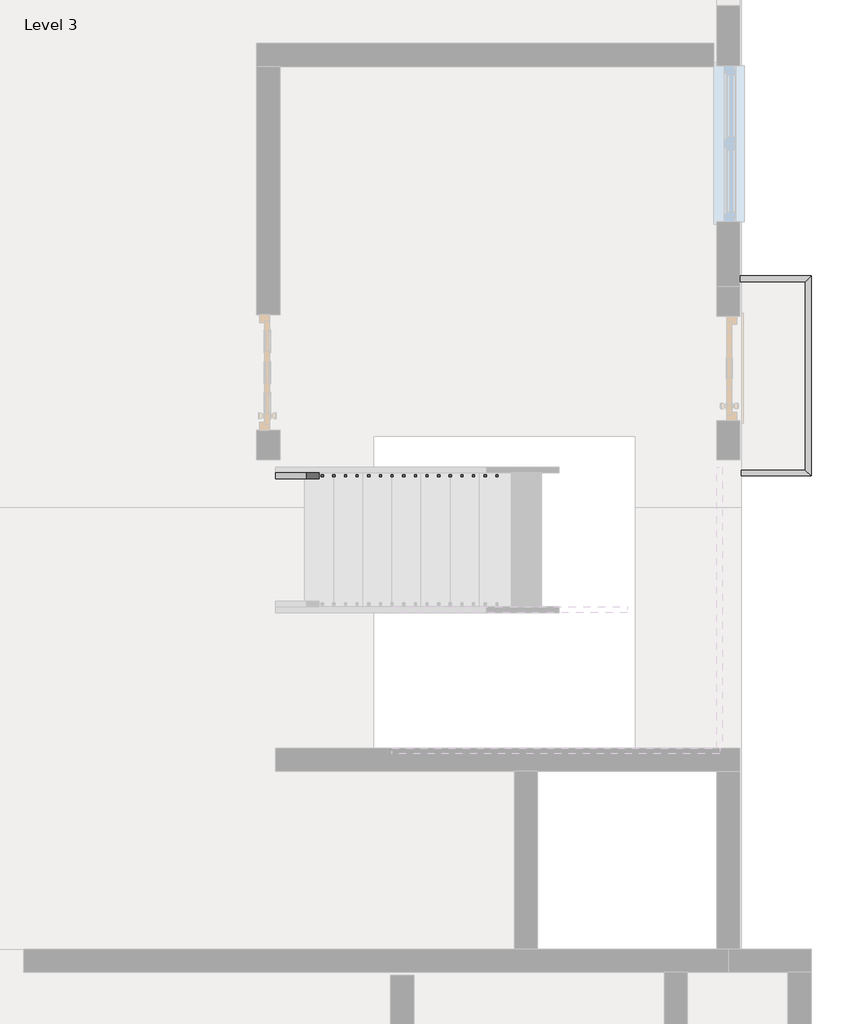
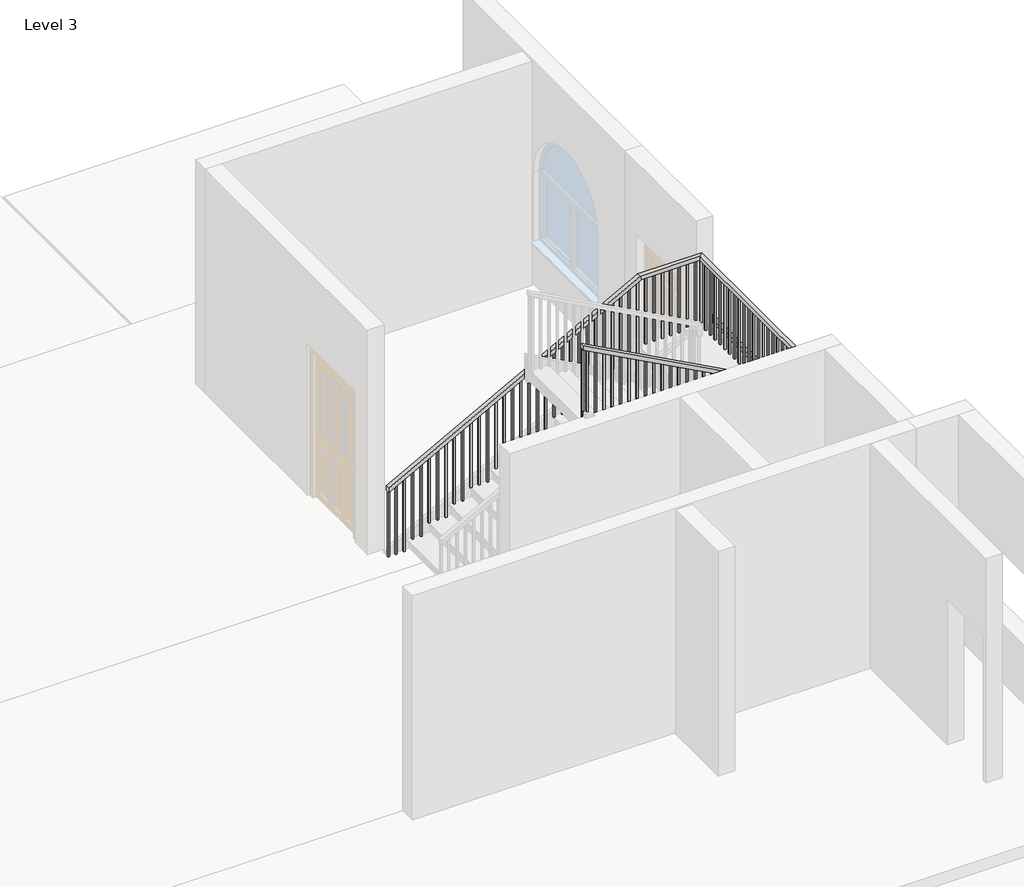
# One storey, part 6 of 7: 2 railings.
"""IFC4 building model written with IfcOpenShell, lengths in millimetres."""

from ifc_helpers import new_model, si_unit, frame, origin, place, context, project, spatial, polyline, outline, extrude, faceted_brep, element, save

model = new_model("IFC4")

# Units and contexts
model_context = context("Model", 3, world=origin())
ifc_project = project(units=[si_unit("LENGTHUNIT", "METRE", prefix="MILLI")], contexts=[model_context])

# Site, building, storey
site = spatial("IfcSite", under=ifc_project)
building = spatial("IfcBuilding", under=site)
storey = spatial("IfcBuildingStorey", under=building, Name="Level 3", Elevation=6096.0)

# Railings
placement = place(None, origin())
element("IfcRailing", 1, ObjectType="Handrail - Rectangular", at=placement, inside=storey, context=model_context, shape_type="SolidModel", body=[
    faceted_brep([(5863.1890963, 3183.81308, 7010.4), (5863.1890963, 3183.81308, 6959.6), (5863.1890963, 3133.01308, 6959.6), (5863.1890963, 3133.01308, 7010.4), (6485.4890963, 3183.81308, 7010.4), (6485.4890963, 3183.81308, 6959.6), (6434.6890963, 3133.01308, 6959.6), (6434.6890963, 3133.01308, 7010.4), (6485.4890963, 1439.3962251, 7010.4), (6485.4890963, 1439.3962251, 6959.6), (6434.6890963, 1490.1962251, 6959.6), (6434.6890963, 1490.1962251, 7010.4), (5875.8890963, 1439.3962251, 7010.4), (5875.8890963, 1490.1962251, 7010.4), (5875.8890963, 1490.1962251, 6959.6), (5875.8890963, 1439.3962251, 6959.6)], [[[0, 1, 2, 3]], [[1, 0, 4, 5]], [[2, 1, 5, 6]], [[3, 2, 6, 7]], [[0, 3, 7, 4]], [[5, 4, 8, 9]], [[6, 5, 9, 10]], [[7, 6, 10, 11]], [[4, 7, 11, 8]], [[12, 13, 14, 15]], [[9, 8, 12, 15]], [[10, 9, 15, 14]], [[11, 10, 14, 13]], [[8, 11, 13, 12]]]),
    extrude(outline(polyline([(5961.6140963, 1474.3212251), (5961.6140963, 1455.2712251), (5942.5640963, 1455.2712251), (5942.5640963, 1474.3212251), (5961.6140963, 1474.3212251)])), frame((0.0, 0.0, 6096.0), z_axis=(0.0, 0.0, 1.0), x_axis=(1.0, 0.0, 0.0)), (0.0, 0.0, 1.0), 863.6),
    extrude(outline(polyline([(6063.2140963, 1474.3212251), (6063.2140963, 1455.2712251), (6044.1640963, 1455.2712251), (6044.1640963, 1474.3212251), (6063.2140963, 1474.3212251)])), frame((0.0, 0.0, 6096.0), z_axis=(0.0, 0.0, 1.0), x_axis=(1.0, 0.0, 0.0)), (0.0, 0.0, 1.0), 863.6),
    extrude(outline(polyline([(6164.8140963, 1474.3212251), (6164.8140963, 1455.2712251), (6145.7640963, 1455.2712251), (6145.7640963, 1474.3212251), (6164.8140963, 1474.3212251)])), frame((0.0, 0.0, 6096.0), z_axis=(0.0, 0.0, 1.0), x_axis=(1.0, 0.0, 0.0)), (0.0, 0.0, 1.0), 863.6),
    extrude(outline(polyline([(6266.4140963, 1474.3212251), (6266.4140963, 1455.2712251), (6247.3640963, 1455.2712251), (6247.3640963, 1474.3212251), (6266.4140963, 1474.3212251)])), frame((0.0, 0.0, 6096.0), z_axis=(0.0, 0.0, 1.0), x_axis=(1.0, 0.0, 0.0)), (0.0, 0.0, 1.0), 863.6),
    extrude(outline(polyline([(6368.0140963, 1474.3212251), (6368.0140963, 1455.2712251), (6348.9640963, 1455.2712251), (6348.9640963, 1474.3212251), (6368.0140963, 1474.3212251)])), frame((0.0, 0.0, 6096.0), z_axis=(0.0, 0.0, 1.0), x_axis=(1.0, 0.0, 0.0)), (0.0, 0.0, 1.0), 863.6),
    extrude(outline(polyline([(6450.5640963, 1542.33808), (6469.6140963, 1542.33808), (6469.6140963, 1523.28808), (6450.5640963, 1523.28808), (6450.5640963, 1542.33808)])), frame((0.0, 0.0, 6096.0), z_axis=(0.0, 0.0, 1.0), x_axis=(1.0, 0.0, 0.0)), (0.0, 0.0, 1.0), 863.6),
    extrude(outline(polyline([(6450.5640963, 1643.93808), (6469.6140963, 1643.93808), (6469.6140963, 1624.88808), (6450.5640963, 1624.88808), (6450.5640963, 1643.93808)])), frame((0.0, 0.0, 6096.0), z_axis=(0.0, 0.0, 1.0), x_axis=(1.0, 0.0, 0.0)), (0.0, 0.0, 1.0), 863.6),
    extrude(outline(polyline([(6450.5640963, 1745.53808), (6469.6140963, 1745.53808), (6469.6140963, 1726.48808), (6450.5640963, 1726.48808), (6450.5640963, 1745.53808)])), frame((0.0, 0.0, 6096.0), z_axis=(0.0, 0.0, 1.0), x_axis=(1.0, 0.0, 0.0)), (0.0, 0.0, 1.0), 863.6),
    extrude(outline(polyline([(6450.5640963, 1847.13808), (6469.6140963, 1847.13808), (6469.6140963, 1828.08808), (6450.5640963, 1828.08808), (6450.5640963, 1847.13808)])), frame((0.0, 0.0, 6096.0), z_axis=(0.0, 0.0, 1.0), x_axis=(1.0, 0.0, 0.0)), (0.0, 0.0, 1.0), 863.6),
    extrude(outline(polyline([(6450.5640963, 1948.73808), (6469.6140963, 1948.73808), (6469.6140963, 1929.68808), (6450.5640963, 1929.68808), (6450.5640963, 1948.73808)])), frame((0.0, 0.0, 6096.0), z_axis=(0.0, 0.0, 1.0), x_axis=(1.0, 0.0, 0.0)), (0.0, 0.0, 1.0), 863.6),
    extrude(outline(polyline([(6450.5640963, 2050.33808), (6469.6140963, 2050.33808), (6469.6140963, 2031.28808), (6450.5640963, 2031.28808), (6450.5640963, 2050.33808)])), frame((0.0, 0.0, 6096.0), z_axis=(0.0, 0.0, 1.0), x_axis=(1.0, 0.0, 0.0)), (0.0, 0.0, 1.0), 863.6),
    extrude(outline(polyline([(6450.5640963, 2151.93808), (6469.6140963, 2151.93808), (6469.6140963, 2132.88808), (6450.5640963, 2132.88808), (6450.5640963, 2151.93808)])), frame((0.0, 0.0, 6096.0), z_axis=(0.0, 0.0, 1.0), x_axis=(1.0, 0.0, 0.0)), (0.0, 0.0, 1.0), 863.6),
    extrude(outline(polyline([(6450.5640963, 2253.53808), (6469.6140963, 2253.53808), (6469.6140963, 2234.48808), (6450.5640963, 2234.48808), (6450.5640963, 2253.53808)])), frame((0.0, 0.0, 6096.0), z_axis=(0.0, 0.0, 1.0), x_axis=(1.0, 0.0, 0.0)), (0.0, 0.0, 1.0), 863.6),
    extrude(outline(polyline([(6450.5640963, 2355.13808), (6469.6140963, 2355.13808), (6469.6140963, 2336.08808), (6450.5640963, 2336.08808), (6450.5640963, 2355.13808)])), frame((0.0, 0.0, 6096.0), z_axis=(0.0, 0.0, 1.0), x_axis=(1.0, 0.0, 0.0)), (0.0, 0.0, 1.0), 863.6),
    extrude(outline(polyline([(6450.5640963, 2456.73808), (6469.6140963, 2456.73808), (6469.6140963, 2437.68808), (6450.5640963, 2437.68808), (6450.5640963, 2456.73808)])), frame((0.0, 0.0, 6096.0), z_axis=(0.0, 0.0, 1.0), x_axis=(1.0, 0.0, 0.0)), (0.0, 0.0, 1.0), 863.6),
    extrude(outline(polyline([(6450.5640963, 2558.33808), (6469.6140963, 2558.33808), (6469.6140963, 2539.28808), (6450.5640963, 2539.28808), (6450.5640963, 2558.33808)])), frame((0.0, 0.0, 6096.0), z_axis=(0.0, 0.0, 1.0), x_axis=(1.0, 0.0, 0.0)), (0.0, 0.0, 1.0), 863.6),
    extrude(outline(polyline([(6450.5640963, 2659.93808), (6469.6140963, 2659.93808), (6469.6140963, 2640.88808), (6450.5640963, 2640.88808), (6450.5640963, 2659.93808)])), frame((0.0, 0.0, 6096.0), z_axis=(0.0, 0.0, 1.0), x_axis=(1.0, 0.0, 0.0)), (0.0, 0.0, 1.0), 863.6),
    extrude(outline(polyline([(6450.5640963, 2761.53808), (6469.6140963, 2761.53808), (6469.6140963, 2742.48808), (6450.5640963, 2742.48808), (6450.5640963, 2761.53808)])), frame((0.0, 0.0, 6096.0), z_axis=(0.0, 0.0, 1.0), x_axis=(1.0, 0.0, 0.0)), (0.0, 0.0, 1.0), 863.6),
    extrude(outline(polyline([(6450.5640963, 2863.13808), (6469.6140963, 2863.13808), (6469.6140963, 2844.08808), (6450.5640963, 2844.08808), (6450.5640963, 2863.13808)])), frame((0.0, 0.0, 6096.0), z_axis=(0.0, 0.0, 1.0), x_axis=(1.0, 0.0, 0.0)), (0.0, 0.0, 1.0), 863.6),
    extrude(outline(polyline([(6450.5640963, 2964.73808), (6469.6140963, 2964.73808), (6469.6140963, 2945.68808), (6450.5640963, 2945.68808), (6450.5640963, 2964.73808)])), frame((0.0, 0.0, 6096.0), z_axis=(0.0, 0.0, 1.0), x_axis=(1.0, 0.0, 0.0)), (0.0, 0.0, 1.0), 863.6),
    extrude(outline(polyline([(6450.5640963, 3066.33808), (6469.6140963, 3066.33808), (6469.6140963, 3047.28808), (6450.5640963, 3047.28808), (6450.5640963, 3066.33808)])), frame((0.0, 0.0, 6096.0), z_axis=(0.0, 0.0, 1.0), x_axis=(1.0, 0.0, 0.0)), (0.0, 0.0, 1.0), 863.6),
    extrude(outline(polyline([(6361.6640963, 3148.88808), (6361.6640963, 3167.93808), (6380.7140963, 3167.93808), (6380.7140963, 3148.88808), (6361.6640963, 3148.88808)])), frame((0.0, 0.0, 6096.0), z_axis=(0.0, 0.0, 1.0), x_axis=(1.0, 0.0, 0.0)), (0.0, 0.0, 1.0), 863.6),
    extrude(outline(polyline([(6260.0640963, 3148.88808), (6260.0640963, 3167.93808), (6279.1140963, 3167.93808), (6279.1140963, 3148.88808), (6260.0640963, 3148.88808)])), frame((0.0, 0.0, 6096.0), z_axis=(0.0, 0.0, 1.0), x_axis=(1.0, 0.0, 0.0)), (0.0, 0.0, 1.0), 863.6),
    extrude(outline(polyline([(6158.4640963, 3148.88808), (6158.4640963, 3167.93808), (6177.5140963, 3167.93808), (6177.5140963, 3148.88808), (6158.4640963, 3148.88808)])), frame((0.0, 0.0, 6096.0), z_axis=(0.0, 0.0, 1.0), x_axis=(1.0, 0.0, 0.0)), (0.0, 0.0, 1.0), 863.6),
    extrude(outline(polyline([(6056.8640963, 3148.88808), (6056.8640963, 3167.93808), (6075.9140963, 3167.93808), (6075.9140963, 3148.88808), (6056.8640963, 3148.88808)])), frame((0.0, 0.0, 6096.0), z_axis=(0.0, 0.0, 1.0), x_axis=(1.0, 0.0, 0.0)), (0.0, 0.0, 1.0), 863.6),
    extrude(outline(polyline([(5955.2640963, 3148.88808), (5955.2640963, 3167.93808), (5974.3140963, 3167.93808), (5974.3140963, 3148.88808), (5955.2640963, 3148.88808)])), frame((0.0, 0.0, 6096.0), z_axis=(0.0, 0.0, 1.0), x_axis=(1.0, 0.0, 0.0)), (0.0, 0.0, 1.0), 863.6),
    extrude(outline(polyline([(6450.5640963, 1474.3212251), (6469.6140963, 1474.3212251), (6469.6140963, 1455.2712251), (6450.5640963, 1455.2712251), (6450.5640963, 1474.3212251)])), frame((0.0, 0.0, 6096.0), z_axis=(0.0, 0.0, 1.0), x_axis=(1.0, 0.0, 0.0)), (0.0, 0.0, 1.0), 863.6),
    extrude(outline(polyline([(6450.5640963, 3148.88808), (6450.5640963, 3167.93808), (6469.6140963, 3167.93808), (6469.6140963, 3148.88808), (6450.5640963, 3148.88808)])), frame((0.0, 0.0, 6096.0), z_axis=(0.0, 0.0, 1.0), x_axis=(1.0, 0.0, 0.0)), (0.0, 0.0, 1.0), 863.6),
    extrude(outline(polyline([(5894.9390963, 1474.3212251), (5894.9390963, 1455.2712251), (5875.8890963, 1455.2712251), (5875.8890963, 1474.3212251), (5894.9390963, 1474.3212251)])), frame((0.0, 0.0, 6096.0), z_axis=(0.0, 0.0, 1.0), x_axis=(1.0, 0.0, 0.0)), (0.0, 0.0, 1.0), 863.6),
    extrude(outline(polyline([(5863.1890963, 3148.88808), (5863.1890963, 3167.93808), (5882.2390963, 3167.93808), (5882.2390963, 3148.88808), (5863.1890963, 3148.88808)])), frame((0.0, 0.0, 6096.0), z_axis=(0.0, 0.0, 1.0), x_axis=(1.0, 0.0, 0.0)), (0.0, 0.0, 1.0), 863.6),
])
element("IfcRailing", 2, ObjectType="Handrail - Rectangular", at=placement, inside=storey, context=model_context, shape_type="SolidModel", body=[
    faceted_brep([(1811.8890963, 1464.7962251, 7148.9454545), (1811.8890963, 1464.7962251, 7091.1709673), (1811.8890963, 1413.9962251, 7091.1709673), (1811.8890963, 1413.9962251, 7148.9454545), (4881.0326586, 1464.7962251, 8811.4909091), (4893.9079172, 1464.7962251, 8760.6909091), (4893.9079172, 1413.9962251, 8760.6909091), (4881.0326586, 1413.9962251, 8811.4909091), (5659.9890963, 1464.7962251, 8811.4909091), (5659.9890963, 1464.7962251, 8760.6909091), (5609.1890963, 1413.9962251, 8760.6909091), (5609.1890963, 1413.9962251, 8811.4909091), (5659.9890963, -935.5037749, 8811.4909091), (5659.9890963, -935.5037749, 8760.6909091), (5609.1890963, -884.7037749, 8760.6909091), (5609.1890963, -884.7037749, 8811.4909091), (5137.6756039, -935.5037749, 8811.4909091), (5124.8392301, -935.5037749, 8760.6909091), (5124.8392301, -884.7037749, 8760.6909091), (5137.6756039, -884.7037749, 8811.4909091), (2827.8890963, -935.5037749, 10058.4), (2827.8890963, -884.7037749, 10058.4), (2827.8890963, -884.7037749, 10000.6704456), (2827.8890963, -935.5037749, 10000.6704456)], [[[0, 1, 2, 3]], [[1, 0, 4, 5]], [[2, 1, 5, 6]], [[3, 2, 6, 7]], [[0, 3, 7, 4]], [[5, 4, 8, 9]], [[6, 5, 9, 10]], [[7, 6, 10, 11]], [[4, 7, 11, 8]], [[9, 8, 12, 13]], [[10, 9, 13, 14]], [[11, 10, 14, 15]], [[8, 11, 15, 12]], [[13, 12, 16, 17]], [[14, 13, 17, 18]], [[15, 14, 18, 19]], [[12, 15, 19, 16]], [[20, 21, 22, 23]], [[17, 16, 20, 23]], [[18, 17, 23, 22]], [[19, 18, 22, 21]], [[16, 19, 21, 20]]]),
    extrude(outline(polyline([(9971.5858236, 2881.8640963), (9005.4545455, 2881.8640963), (9005.4545455, 2900.9140963), (9961.2664983, 2900.9140963), (9971.5858236, 2881.8640963)])), frame((0.0, -919.6287749, 0.0), z_axis=(0.0, 1.0, 0.0), x_axis=(0.0, 0.0, 1.0)), (0.0, 0.0, 1.0), 19.05),
    extrude(outline(polyline([(9916.5494219, 2983.4640963), (9005.4545455, 2983.4640963), (9005.4545455, 3002.5140963), (9906.2300965, 3002.5140963), (9916.5494219, 2983.4640963)])), frame((0.0, -919.6287749, 0.0), z_axis=(0.0, 1.0, 0.0), x_axis=(0.0, 0.0, 1.0)), (0.0, 0.0, 1.0), 19.05),
    extrude(outline(polyline([(9861.8377681, 3085.0640963), (8866.9090909, 3085.0640963), (8866.9090909, 3104.1140963), (9851.553866, 3104.1140963), (9861.8377681, 3085.0640963)])), frame((0.0, -919.6287749, 0.0), z_axis=(0.0, 1.0, 0.0), x_axis=(0.0, 0.0, 1.0)), (0.0, 0.0, 1.0), 19.05),
    extrude(outline(polyline([(9806.9902905, 3186.6640963), (8866.9090909, 3186.6640963), (8866.9090909, 3205.7140963), (9796.7063885, 3205.7140963), (9806.9902905, 3186.6640963)])), frame((0.0, -919.6287749, 0.0), z_axis=(0.0, 1.0, 0.0), x_axis=(0.0, 0.0, 1.0)), (0.0, 0.0, 1.0), 19.05),
    extrude(outline(polyline([(9752.1428129, 3288.2640963), (8866.9090909, 3288.2640963), (8866.9090909, 3307.3140963), (9741.8589109, 3307.3140963), (9752.1428129, 3288.2640963)])), frame((0.0, -919.6287749, 0.0), z_axis=(0.0, 1.0, 0.0), x_axis=(0.0, 0.0, 1.0)), (0.0, 0.0, 1.0), 19.05),
    extrude(outline(polyline([(9697.2953354, 3389.8640963), (8728.3636364, 3389.8640963), (8728.3636364, 3408.9140963), (9687.0114333, 3408.9140963), (9697.2953354, 3389.8640963)])), frame((0.0, -919.6287749, 0.0), z_axis=(0.0, 1.0, 0.0), x_axis=(0.0, 0.0, 1.0)), (0.0, 0.0, 1.0), 19.05),
    extrude(outline(polyline([(9642.4478578, 3491.4640963), (8728.3636364, 3491.4640963), (8728.3636364, 3510.5140963), (9632.1639558, 3510.5140963), (9642.4478578, 3491.4640963)])), frame((0.0, -919.6287749, 0.0), z_axis=(0.0, 1.0, 0.0), x_axis=(0.0, 0.0, 1.0)), (0.0, 0.0, 1.0), 19.05),
    extrude(outline(polyline([(9587.6003803, 3593.0640963), (8589.8181818, 3593.0640963), (8589.8181818, 3612.1140963), (9577.3164782, 3612.1140963), (9587.6003803, 3593.0640963)])), frame((0.0, -919.6287749, 0.0), z_axis=(0.0, 1.0, 0.0), x_axis=(0.0, 0.0, 1.0)), (0.0, 0.0, 1.0), 19.05),
    extrude(outline(polyline([(9532.7529027, 3694.6640963), (8589.8181818, 3694.6640963), (8589.8181818, 3713.7140963), (9522.4690007, 3713.7140963), (9532.7529027, 3694.6640963)])), frame((0.0, -919.6287749, 0.0), z_axis=(0.0, 1.0, 0.0), x_axis=(0.0, 0.0, 1.0)), (0.0, 0.0, 1.0), 19.05),
    extrude(outline(polyline([(9477.9054252, 3796.2640963), (8589.8181818, 3796.2640963), (8589.8181818, 3815.3140963), (9467.6215231, 3815.3140963), (9477.9054252, 3796.2640963)])), frame((0.0, -919.6287749, 0.0), z_axis=(0.0, 1.0, 0.0), x_axis=(0.0, 0.0, 1.0)), (0.0, 0.0, 1.0), 19.05),
    extrude(outline(polyline([(9423.1307062, 3897.8640963), (8451.2727273, 3897.8640963), (8451.2727273, 3916.9140963), (9412.8113809, 3916.9140963), (9423.1307062, 3897.8640963)])), frame((0.0, -919.6287749, 0.0), z_axis=(0.0, 1.0, 0.0), x_axis=(0.0, 0.0, 1.0)), (0.0, 0.0, 1.0), 19.05),
    extrude(outline(polyline([(9368.0943044, 3999.4640963), (8451.2727273, 3999.4640963), (8451.2727273, 4018.5140963), (9357.7749791, 4018.5140963), (9368.0943044, 3999.4640963)])), frame((0.0, -919.6287749, 0.0), z_axis=(0.0, 1.0, 0.0), x_axis=(0.0, 0.0, 1.0)), (0.0, 0.0, 1.0), 19.05),
    extrude(outline(polyline([(9313.3629925, 4101.0640963), (8312.7272727, 4101.0640963), (8312.7272727, 4120.1140963), (9303.0790904, 4120.1140963), (9313.3629925, 4101.0640963)])), frame((0.0, -919.6287749, 0.0), z_axis=(0.0, 1.0, 0.0), x_axis=(0.0, 0.0, 1.0)), (0.0, 0.0, 1.0), 19.05),
    extrude(outline(polyline([(9258.5155149, 4202.6640963), (8312.7272727, 4202.6640963), (8312.7272727, 4221.7140963), (9248.2316129, 4221.7140963), (9258.5155149, 4202.6640963)])), frame((0.0, -919.6287749, 0.0), z_axis=(0.0, 1.0, 0.0), x_axis=(0.0, 0.0, 1.0)), (0.0, 0.0, 1.0), 19.05),
    extrude(outline(polyline([(9203.6680374, 4304.2640963), (8312.7272727, 4304.2640963), (8312.7272727, 4323.3140963), (9193.3841353, 4323.3140963), (9203.6680374, 4304.2640963)])), frame((0.0, -919.6287749, 0.0), z_axis=(0.0, 1.0, 0.0), x_axis=(0.0, 0.0, 1.0)), (0.0, 0.0, 1.0), 19.05),
    extrude(outline(polyline([(9148.8205598, 4405.8640963), (8174.1818182, 4405.8640963), (8174.1818182, 4424.9140963), (9138.5366578, 4424.9140963), (9148.8205598, 4405.8640963)])), frame((0.0, -919.6287749, 0.0), z_axis=(0.0, 1.0, 0.0), x_axis=(0.0, 0.0, 1.0)), (0.0, 0.0, 1.0), 19.05),
    extrude(outline(polyline([(9093.9730823, 4507.4640963), (8174.1818182, 4507.4640963), (8174.1818182, 4526.5140963), (9083.6891802, 4526.5140963), (9093.9730823, 4507.4640963)])), frame((0.0, -919.6287749, 0.0), z_axis=(0.0, 1.0, 0.0), x_axis=(0.0, 0.0, 1.0)), (0.0, 0.0, 1.0), 19.05),
    extrude(outline(polyline([(9039.1256047, 4609.0640963), (8035.6363636, 4609.0640963), (8035.6363636, 4628.1140963), (9028.8417027, 4628.1140963), (9039.1256047, 4609.0640963)])), frame((0.0, -919.6287749, 0.0), z_axis=(0.0, 1.0, 0.0), x_axis=(0.0, 0.0, 1.0)), (0.0, 0.0, 1.0), 19.05),
    extrude(outline(polyline([(8984.2781272, 4710.6640963), (8035.6363636, 4710.6640963), (8035.6363636, 4729.7140963), (8973.9942251, 4729.7140963), (8984.2781272, 4710.6640963)])), frame((0.0, -919.6287749, 0.0), z_axis=(0.0, 1.0, 0.0), x_axis=(0.0, 0.0, 1.0)), (0.0, 0.0, 1.0), 19.05),
    extrude(outline(polyline([(8929.4306496, 4812.2640963), (8035.6363636, 4812.2640963), (8035.6363636, 4831.3140963), (8919.1467476, 4831.3140963), (8929.4306496, 4812.2640963)])), frame((0.0, -919.6287749, 0.0), z_axis=(0.0, 1.0, 0.0), x_axis=(0.0, 0.0, 1.0)), (0.0, 0.0, 1.0), 19.05),
    extrude(outline(polyline([(8874.583172, 4913.8640963), (7897.0909091, 4913.8640963), (7897.0909091, 4932.9140963), (8864.29927, 4932.9140963), (8874.583172, 4913.8640963)])), frame((0.0, -919.6287749, 0.0), z_axis=(0.0, 1.0, 0.0), x_axis=(0.0, 0.0, 1.0)), (0.0, 0.0, 1.0), 19.05),
    extrude(outline(polyline([(8819.7356945, 5015.4640963), (7897.0909091, 5015.4640963), (7897.0909091, 5034.5140963), (8809.4517924, 5034.5140963), (8819.7356945, 5015.4640963)])), frame((0.0, -919.6287749, 0.0), z_axis=(0.0, 1.0, 0.0), x_axis=(0.0, 0.0, 1.0)), (0.0, 0.0, 1.0), 19.05),
    extrude(outline(polyline([(8764.8882169, 5117.0640963), (7897.0909091, 5117.0640963), (7897.0909091, 5136.1140963), (8754.6043149, 5136.1140963), (8764.8882169, 5117.0640963)])), frame((0.0, -919.6287749, 0.0), z_axis=(0.0, 1.0, 0.0), x_axis=(0.0, 0.0, 1.0)), (0.0, 0.0, 1.0), 19.05),
    extrude(outline(polyline([(5237.7140963, -919.6287749), (5218.6640963, -919.6287749), (5218.6640963, -900.5787749), (5237.7140963, -900.5787749), (5237.7140963, -919.6287749)])), frame((0.0, 0.0, 7897.0909091), z_axis=(0.0, 0.0, 1.0), x_axis=(1.0, 0.0, 0.0)), (0.0, 0.0, 1.0), 863.6),
    extrude(outline(polyline([(5339.3140963, -919.6287749), (5320.2640963, -919.6287749), (5320.2640963, -900.5787749), (5339.3140963, -900.5787749), (5339.3140963, -919.6287749)])), frame((0.0, 0.0, 7897.0909091), z_axis=(0.0, 0.0, 1.0), x_axis=(1.0, 0.0, 0.0)), (0.0, 0.0, 1.0), 863.6),
    extrude(outline(polyline([(5440.9140963, -919.6287749), (5421.8640963, -919.6287749), (5421.8640963, -900.5787749), (5440.9140963, -900.5787749), (5440.9140963, -919.6287749)])), frame((0.0, 0.0, 7897.0909091), z_axis=(0.0, 0.0, 1.0), x_axis=(1.0, 0.0, 0.0)), (0.0, 0.0, 1.0), 863.6),
    extrude(outline(polyline([(5542.5140963, -919.6287749), (5523.4640963, -919.6287749), (5523.4640963, -900.5787749), (5542.5140963, -900.5787749), (5542.5140963, -919.6287749)])), frame((0.0, 0.0, 7897.0909091), z_axis=(0.0, 0.0, 1.0), x_axis=(1.0, 0.0, 0.0)), (0.0, 0.0, 1.0), 863.6),
    extrude(outline(polyline([(5644.1140963, -887.8787749), (5644.1140963, -906.9287749), (5625.0640963, -906.9287749), (5625.0640963, -887.8787749), (5644.1140963, -887.8787749)])), frame((0.0, 0.0, 7897.0909091), z_axis=(0.0, 0.0, 1.0), x_axis=(1.0, 0.0, 0.0)), (0.0, 0.0, 1.0), 863.6),
    extrude(outline(polyline([(5644.1140963, -786.2787749), (5644.1140963, -805.3287749), (5625.0640963, -805.3287749), (5625.0640963, -786.2787749), (5644.1140963, -786.2787749)])), frame((0.0, 0.0, 7897.0909091), z_axis=(0.0, 0.0, 1.0), x_axis=(1.0, 0.0, 0.0)), (0.0, 0.0, 1.0), 863.6),
    extrude(outline(polyline([(5644.1140963, -684.6787749), (5644.1140963, -703.7287749), (5625.0640963, -703.7287749), (5625.0640963, -684.6787749), (5644.1140963, -684.6787749)])), frame((0.0, 0.0, 7897.0909091), z_axis=(0.0, 0.0, 1.0), x_axis=(1.0, 0.0, 0.0)), (0.0, 0.0, 1.0), 863.6),
    extrude(outline(polyline([(5644.1140963, -583.0787749), (5644.1140963, -602.1287749), (5625.0640963, -602.1287749), (5625.0640963, -583.0787749), (5644.1140963, -583.0787749)])), frame((0.0, 0.0, 7897.0909091), z_axis=(0.0, 0.0, 1.0), x_axis=(1.0, 0.0, 0.0)), (0.0, 0.0, 1.0), 863.6),
    extrude(outline(polyline([(5644.1140963, -481.4787749), (5644.1140963, -500.5287749), (5625.0640963, -500.5287749), (5625.0640963, -481.4787749), (5644.1140963, -481.4787749)])), frame((0.0, 0.0, 7897.0909091), z_axis=(0.0, 0.0, 1.0), x_axis=(1.0, 0.0, 0.0)), (0.0, 0.0, 1.0), 863.6),
    extrude(outline(polyline([(5644.1140963, -379.8787749), (5644.1140963, -398.9287749), (5625.0640963, -398.9287749), (5625.0640963, -379.8787749), (5644.1140963, -379.8787749)])), frame((0.0, 0.0, 7897.0909091), z_axis=(0.0, 0.0, 1.0), x_axis=(1.0, 0.0, 0.0)), (0.0, 0.0, 1.0), 863.6),
    extrude(outline(polyline([(5644.1140963, -278.2787749), (5644.1140963, -297.3287749), (5625.0640963, -297.3287749), (5625.0640963, -278.2787749), (5644.1140963, -278.2787749)])), frame((0.0, 0.0, 7897.0909091), z_axis=(0.0, 0.0, 1.0), x_axis=(1.0, 0.0, 0.0)), (0.0, 0.0, 1.0), 863.6),
    extrude(outline(polyline([(5644.1140963, -176.6787749), (5644.1140963, -195.7287749), (5625.0640963, -195.7287749), (5625.0640963, -176.6787749), (5644.1140963, -176.6787749)])), frame((0.0, 0.0, 7897.0909091), z_axis=(0.0, 0.0, 1.0), x_axis=(1.0, 0.0, 0.0)), (0.0, 0.0, 1.0), 863.6),
    extrude(outline(polyline([(5644.1140963, -75.0787749), (5644.1140963, -94.1287749), (5625.0640963, -94.1287749), (5625.0640963, -75.0787749), (5644.1140963, -75.0787749)])), frame((0.0, 0.0, 7897.0909091), z_axis=(0.0, 0.0, 1.0), x_axis=(1.0, 0.0, 0.0)), (0.0, 0.0, 1.0), 863.6),
    extrude(outline(polyline([(5644.1140963, 26.5212251), (5644.1140963, 7.4712251), (5625.0640963, 7.4712251), (5625.0640963, 26.5212251), (5644.1140963, 26.5212251)])), frame((0.0, 0.0, 7897.0909091), z_axis=(0.0, 0.0, 1.0), x_axis=(1.0, 0.0, 0.0)), (0.0, 0.0, 1.0), 863.6),
    extrude(outline(polyline([(5644.1140963, 128.1212251), (5644.1140963, 109.0712251), (5625.0640963, 109.0712251), (5625.0640963, 128.1212251), (5644.1140963, 128.1212251)])), frame((0.0, 0.0, 7897.0909091), z_axis=(0.0, 0.0, 1.0), x_axis=(1.0, 0.0, 0.0)), (0.0, 0.0, 1.0), 863.6),
    extrude(outline(polyline([(5644.1140963, 229.7212251), (5644.1140963, 210.6712251), (5625.0640963, 210.6712251), (5625.0640963, 229.7212251), (5644.1140963, 229.7212251)])), frame((0.0, 0.0, 7897.0909091), z_axis=(0.0, 0.0, 1.0), x_axis=(1.0, 0.0, 0.0)), (0.0, 0.0, 1.0), 863.6),
    extrude(outline(polyline([(5644.1140963, 331.3212251), (5644.1140963, 312.2712251), (5625.0640963, 312.2712251), (5625.0640963, 331.3212251), (5644.1140963, 331.3212251)])), frame((0.0, 0.0, 7897.0909091), z_axis=(0.0, 0.0, 1.0), x_axis=(1.0, 0.0, 0.0)), (0.0, 0.0, 1.0), 863.6),
    extrude(outline(polyline([(5644.1140963, 432.9212251), (5644.1140963, 413.8712251), (5625.0640963, 413.8712251), (5625.0640963, 432.9212251), (5644.1140963, 432.9212251)])), frame((0.0, 0.0, 7897.0909091), z_axis=(0.0, 0.0, 1.0), x_axis=(1.0, 0.0, 0.0)), (0.0, 0.0, 1.0), 863.6),
    extrude(outline(polyline([(5644.1140963, 534.5212251), (5644.1140963, 515.4712251), (5625.0640963, 515.4712251), (5625.0640963, 534.5212251), (5644.1140963, 534.5212251)])), frame((0.0, 0.0, 7897.0909091), z_axis=(0.0, 0.0, 1.0), x_axis=(1.0, 0.0, 0.0)), (0.0, 0.0, 1.0), 863.6),
    extrude(outline(polyline([(5644.1140963, 636.1212251), (5644.1140963, 617.0712251), (5625.0640963, 617.0712251), (5625.0640963, 636.1212251), (5644.1140963, 636.1212251)])), frame((0.0, 0.0, 7897.0909091), z_axis=(0.0, 0.0, 1.0), x_axis=(1.0, 0.0, 0.0)), (0.0, 0.0, 1.0), 863.6),
    extrude(outline(polyline([(5644.1140963, 737.7212251), (5644.1140963, 718.6712251), (5625.0640963, 718.6712251), (5625.0640963, 737.7212251), (5644.1140963, 737.7212251)])), frame((0.0, 0.0, 7897.0909091), z_axis=(0.0, 0.0, 1.0), x_axis=(1.0, 0.0, 0.0)), (0.0, 0.0, 1.0), 863.6),
    extrude(outline(polyline([(5644.1140963, 839.3212251), (5644.1140963, 820.2712251), (5625.0640963, 820.2712251), (5625.0640963, 839.3212251), (5644.1140963, 839.3212251)])), frame((0.0, 0.0, 7897.0909091), z_axis=(0.0, 0.0, 1.0), x_axis=(1.0, 0.0, 0.0)), (0.0, 0.0, 1.0), 863.6),
    extrude(outline(polyline([(5644.1140963, 940.9212251), (5644.1140963, 921.8712251), (5625.0640963, 921.8712251), (5625.0640963, 940.9212251), (5644.1140963, 940.9212251)])), frame((0.0, 0.0, 7897.0909091), z_axis=(0.0, 0.0, 1.0), x_axis=(1.0, 0.0, 0.0)), (0.0, 0.0, 1.0), 863.6),
    extrude(outline(polyline([(5644.1140963, 1042.5212251), (5644.1140963, 1023.4712251), (5625.0640963, 1023.4712251), (5625.0640963, 1042.5212251), (5644.1140963, 1042.5212251)])), frame((0.0, 0.0, 7897.0909091), z_axis=(0.0, 0.0, 1.0), x_axis=(1.0, 0.0, 0.0)), (0.0, 0.0, 1.0), 863.6),
    extrude(outline(polyline([(5644.1140963, 1144.1212251), (5644.1140963, 1125.0712251), (5625.0640963, 1125.0712251), (5625.0640963, 1144.1212251), (5644.1140963, 1144.1212251)])), frame((0.0, 0.0, 7897.0909091), z_axis=(0.0, 0.0, 1.0), x_axis=(1.0, 0.0, 0.0)), (0.0, 0.0, 1.0), 863.6),
    extrude(outline(polyline([(5644.1140963, 1245.7212251), (5644.1140963, 1226.6712251), (5625.0640963, 1226.6712251), (5625.0640963, 1245.7212251), (5644.1140963, 1245.7212251)])), frame((0.0, 0.0, 7897.0909091), z_axis=(0.0, 0.0, 1.0), x_axis=(1.0, 0.0, 0.0)), (0.0, 0.0, 1.0), 863.6),
    extrude(outline(polyline([(5644.1140963, 1347.3212251), (5644.1140963, 1328.2712251), (5625.0640963, 1328.2712251), (5625.0640963, 1347.3212251), (5644.1140963, 1347.3212251)])), frame((0.0, 0.0, 7897.0909091), z_axis=(0.0, 0.0, 1.0), x_axis=(1.0, 0.0, 0.0)), (0.0, 0.0, 1.0), 863.6),
    extrude(outline(polyline([(5561.5640963, 1448.9212251), (5580.6140963, 1448.9212251), (5580.6140963, 1429.8712251), (5561.5640963, 1429.8712251), (5561.5640963, 1448.9212251)])), frame((0.0, 0.0, 7897.0909091), z_axis=(0.0, 0.0, 1.0), x_axis=(1.0, 0.0, 0.0)), (0.0, 0.0, 1.0), 863.6),
    extrude(outline(polyline([(5459.9640963, 1448.9212251), (5479.0140963, 1448.9212251), (5479.0140963, 1429.8712251), (5459.9640963, 1429.8712251), (5459.9640963, 1448.9212251)])), frame((0.0, 0.0, 7897.0909091), z_axis=(0.0, 0.0, 1.0), x_axis=(1.0, 0.0, 0.0)), (0.0, 0.0, 1.0), 863.6),
    extrude(outline(polyline([(5358.3640963, 1448.9212251), (5377.4140963, 1448.9212251), (5377.4140963, 1429.8712251), (5358.3640963, 1429.8712251), (5358.3640963, 1448.9212251)])), frame((0.0, 0.0, 7897.0909091), z_axis=(0.0, 0.0, 1.0), x_axis=(1.0, 0.0, 0.0)), (0.0, 0.0, 1.0), 863.6),
    extrude(outline(polyline([(5256.7640963, 1448.9212251), (5275.8140963, 1448.9212251), (5275.8140963, 1429.8712251), (5256.7640963, 1429.8712251), (5256.7640963, 1448.9212251)])), frame((0.0, 0.0, 7897.0909091), z_axis=(0.0, 0.0, 1.0), x_axis=(1.0, 0.0, 0.0)), (0.0, 0.0, 1.0), 863.6),
    extrude(outline(polyline([(5155.1640963, 1448.9212251), (5174.2140963, 1448.9212251), (5174.2140963, 1429.8712251), (5155.1640963, 1429.8712251), (5155.1640963, 1448.9212251)])), frame((0.0, 0.0, 7897.0909091), z_axis=(0.0, 0.0, 1.0), x_axis=(1.0, 0.0, 0.0)), (0.0, 0.0, 1.0), 863.6),
    extrude(outline(polyline([(5053.5640963, 1448.9212251), (5072.6140963, 1448.9212251), (5072.6140963, 1429.8712251), (5053.5640963, 1429.8712251), (5053.5640963, 1448.9212251)])), frame((0.0, 0.0, 7897.0909091), z_axis=(0.0, 0.0, 1.0), x_axis=(1.0, 0.0, 0.0)), (0.0, 0.0, 1.0), 863.6),
    extrude(outline(polyline([(4951.9640963, 1448.9212251), (4971.0140963, 1448.9212251), (4971.0140963, 1429.8712251), (4951.9640963, 1429.8712251), (4951.9640963, 1448.9212251)])), frame((0.0, 0.0, 7897.0909091), z_axis=(0.0, 0.0, 1.0), x_axis=(1.0, 0.0, 0.0)), (0.0, 0.0, 1.0), 863.6),
    extrude(outline(polyline([(8737.1033577, 4850.3640963), (7758.5454545, 4850.3640963), (7758.5454545, 4869.4140963), (8747.422683, 4869.4140963), (8737.1033577, 4850.3640963)])), frame((0.0, 1429.8712251, 0.0), z_axis=(0.0, 1.0, 0.0), x_axis=(0.0, 0.0, 1.0)), (0.0, 0.0, 1.0), 19.05),
    extrude(outline(polyline([(8682.0669559, 4748.7640963), (7758.5454545, 4748.7640963), (7758.5454545, 4767.8140963), (8692.3862812, 4767.8140963), (8682.0669559, 4748.7640963)])), frame((0.0, 1429.8712251, 0.0), z_axis=(0.0, 1.0, 0.0), x_axis=(0.0, 0.0, 1.0)), (0.0, 0.0, 1.0), 19.05),
    extrude(outline(polyline([(8627.0305541, 4647.1640963), (7758.5454545, 4647.1640963), (7758.5454545, 4666.2140963), (8637.3498795, 4666.2140963), (8627.0305541, 4647.1640963)])), frame((0.0, 1429.8712251, 0.0), z_axis=(0.0, 1.0, 0.0), x_axis=(0.0, 0.0, 1.0)), (0.0, 0.0, 1.0), 19.05),
    extrude(outline(polyline([(8571.9941524, 4545.5640963), (7620.0, 4545.5640963), (7620.0, 4564.6140963), (8582.3134777, 4564.6140963), (8571.9941524, 4545.5640963)])), frame((0.0, 1429.8712251, 0.0), z_axis=(0.0, 1.0, 0.0), x_axis=(0.0, 0.0, 1.0)), (0.0, 0.0, 1.0), 19.05),
    extrude(outline(polyline([(8516.9577506, 4443.9640963), (7620.0, 4443.9640963), (7620.0, 4463.0140963), (8527.2770759, 4463.0140963), (8516.9577506, 4443.9640963)])), frame((0.0, 1429.8712251, 0.0), z_axis=(0.0, 1.0, 0.0), x_axis=(0.0, 0.0, 1.0)), (0.0, 0.0, 1.0), 19.05),
    extrude(outline(polyline([(8461.9213488, 4342.3640963), (7620.0, 4342.3640963), (7620.0, 4361.4140963), (8472.2406742, 4361.4140963), (8461.9213488, 4342.3640963)])), frame((0.0, 1429.8712251, 0.0), z_axis=(0.0, 1.0, 0.0), x_axis=(0.0, 0.0, 1.0)), (0.0, 0.0, 1.0), 19.05),
    extrude(outline(polyline([(8406.8849471, 4240.7640963), (7481.4545455, 4240.7640963), (7481.4545455, 4259.8140963), (8417.2042724, 4259.8140963), (8406.8849471, 4240.7640963)])), frame((0.0, 1429.8712251, 0.0), z_axis=(0.0, 1.0, 0.0), x_axis=(0.0, 0.0, 1.0)), (0.0, 0.0, 1.0), 19.05),
    extrude(outline(polyline([(8351.8485453, 4139.1640963), (7481.4545455, 4139.1640963), (7481.4545455, 4158.2140963), (8362.1678706, 4158.2140963), (8351.8485453, 4139.1640963)])), frame((0.0, 1429.8712251, 0.0), z_axis=(0.0, 1.0, 0.0), x_axis=(0.0, 0.0, 1.0)), (0.0, 0.0, 1.0), 19.05),
    extrude(outline(polyline([(8296.8121435, 4037.5640963), (7342.9090909, 4037.5640963), (7342.9090909, 4056.6140963), (8307.1314688, 4056.6140963), (8296.8121435, 4037.5640963)])), frame((0.0, 1429.8712251, 0.0), z_axis=(0.0, 1.0, 0.0), x_axis=(0.0, 0.0, 1.0)), (0.0, 0.0, 1.0), 19.05),
    extrude(outline(polyline([(8241.7757417, 3935.9640963), (7342.9090909, 3935.9640963), (7342.9090909, 3955.0140963), (8252.0950671, 3955.0140963), (8241.7757417, 3935.9640963)])), frame((0.0, 1429.8712251, 0.0), z_axis=(0.0, 1.0, 0.0), x_axis=(0.0, 0.0, 1.0)), (0.0, 0.0, 1.0), 19.05),
    extrude(outline(polyline([(8186.73934, 3834.3640963), (7342.9090909, 3834.3640963), (7342.9090909, 3853.4140963), (8197.0586653, 3853.4140963), (8186.73934, 3834.3640963)])), frame((0.0, 1429.8712251, 0.0), z_axis=(0.0, 1.0, 0.0), x_axis=(0.0, 0.0, 1.0)), (0.0, 0.0, 1.0), 19.05),
    extrude(outline(polyline([(8131.7029382, 3732.7640963), (7204.3636364, 3732.7640963), (7204.3636364, 3751.8140963), (8142.0222635, 3751.8140963), (8131.7029382, 3732.7640963)])), frame((0.0, 1429.8712251, 0.0), z_axis=(0.0, 1.0, 0.0), x_axis=(0.0, 0.0, 1.0)), (0.0, 0.0, 1.0), 19.05),
    extrude(outline(polyline([(8076.6665364, 3631.1640963), (7204.3636364, 3631.1640963), (7204.3636364, 3650.2140963), (8086.9858618, 3650.2140963), (8076.6665364, 3631.1640963)])), frame((0.0, 1429.8712251, 0.0), z_axis=(0.0, 1.0, 0.0), x_axis=(0.0, 0.0, 1.0)), (0.0, 0.0, 1.0), 19.05),
    extrude(outline(polyline([(8021.6301347, 3529.5640963), (7065.8181818, 3529.5640963), (7065.8181818, 3548.6140963), (8031.94946, 3548.6140963), (8021.6301347, 3529.5640963)])), frame((0.0, 1429.8712251, 0.0), z_axis=(0.0, 1.0, 0.0), x_axis=(0.0, 0.0, 1.0)), (0.0, 0.0, 1.0), 19.05),
    extrude(outline(polyline([(7966.5937329, 3427.9640963), (7065.8181818, 3427.9640963), (7065.8181818, 3447.0140963), (7976.9130582, 3447.0140963), (7966.5937329, 3427.9640963)])), frame((0.0, 1429.8712251, 0.0), z_axis=(0.0, 1.0, 0.0), x_axis=(0.0, 0.0, 1.0)), (0.0, 0.0, 1.0), 19.05),
    extrude(outline(polyline([(7911.5573311, 3326.3640963), (7065.8181818, 3326.3640963), (7065.8181818, 3345.4140963), (7921.8766565, 3345.4140963), (7911.5573311, 3326.3640963)])), frame((0.0, 1429.8712251, 0.0), z_axis=(0.0, 1.0, 0.0), x_axis=(0.0, 0.0, 1.0)), (0.0, 0.0, 1.0), 19.05),
    extrude(outline(polyline([(7856.5209294, 3224.7640963), (6927.2727273, 3224.7640963), (6927.2727273, 3243.8140963), (7866.8402547, 3243.8140963), (7856.5209294, 3224.7640963)])), frame((0.0, 1429.8712251, 0.0), z_axis=(0.0, 1.0, 0.0), x_axis=(0.0, 0.0, 1.0)), (0.0, 0.0, 1.0), 19.05),
    extrude(outline(polyline([(7801.4845276, 3123.1640963), (6927.2727273, 3123.1640963), (6927.2727273, 3142.2140963), (7811.8038529, 3142.2140963), (7801.4845276, 3123.1640963)])), frame((0.0, 1429.8712251, 0.0), z_axis=(0.0, 1.0, 0.0), x_axis=(0.0, 0.0, 1.0)), (0.0, 0.0, 1.0), 19.05),
    extrude(outline(polyline([(7746.4481258, 3021.5640963), (6788.7272727, 3021.5640963), (6788.7272727, 3040.6140963), (7756.7674512, 3040.6140963), (7746.4481258, 3021.5640963)])), frame((0.0, 1429.8712251, 0.0), z_axis=(0.0, 1.0, 0.0), x_axis=(0.0, 0.0, 1.0)), (0.0, 0.0, 1.0), 19.05),
    extrude(outline(polyline([(7691.4117241, 2919.9640963), (6788.7272727, 2919.9640963), (6788.7272727, 2939.0140963), (7701.7310494, 2939.0140963), (7691.4117241, 2919.9640963)])), frame((0.0, 1429.8712251, 0.0), z_axis=(0.0, 1.0, 0.0), x_axis=(0.0, 0.0, 1.0)), (0.0, 0.0, 1.0), 19.05),
    extrude(outline(polyline([(7636.3753223, 2818.3640963), (6788.7272727, 2818.3640963), (6788.7272727, 2837.4140963), (7646.6946476, 2837.4140963), (7636.3753223, 2818.3640963)])), frame((0.0, 1429.8712251, 0.0), z_axis=(0.0, 1.0, 0.0), x_axis=(0.0, 0.0, 1.0)), (0.0, 0.0, 1.0), 19.05),
    extrude(outline(polyline([(7581.3389205, 2716.7640963), (6650.1818182, 2716.7640963), (6650.1818182, 2735.8140963), (7591.6582459, 2735.8140963), (7581.3389205, 2716.7640963)])), frame((0.0, 1429.8712251, 0.0), z_axis=(0.0, 1.0, 0.0), x_axis=(0.0, 0.0, 1.0)), (0.0, 0.0, 1.0), 19.05),
    extrude(outline(polyline([(7526.3025188, 2615.1640963), (6650.1818182, 2615.1640963), (6650.1818182, 2634.2140963), (7536.6218441, 2634.2140963), (7526.3025188, 2615.1640963)])), frame((0.0, 1429.8712251, 0.0), z_axis=(0.0, 1.0, 0.0), x_axis=(0.0, 0.0, 1.0)), (0.0, 0.0, 1.0), 19.05),
    extrude(outline(polyline([(7471.266117, 2513.5640963), (6511.6363636, 2513.5640963), (6511.6363636, 2532.6140963), (7481.5854423, 2532.6140963), (7471.266117, 2513.5640963)])), frame((0.0, 1429.8712251, 0.0), z_axis=(0.0, 1.0, 0.0), x_axis=(0.0, 0.0, 1.0)), (0.0, 0.0, 1.0), 19.05),
    extrude(outline(polyline([(7416.2297152, 2411.9640963), (6511.6363636, 2411.9640963), (6511.6363636, 2431.0140963), (7426.5490405, 2431.0140963), (7416.2297152, 2411.9640963)])), frame((0.0, 1429.8712251, 0.0), z_axis=(0.0, 1.0, 0.0), x_axis=(0.0, 0.0, 1.0)), (0.0, 0.0, 1.0), 19.05),
    extrude(outline(polyline([(7361.1933134, 2310.3640963), (6511.6363636, 2310.3640963), (6511.6363636, 2329.4140963), (7371.5126388, 2329.4140963), (7361.1933134, 2310.3640963)])), frame((0.0, 1429.8712251, 0.0), z_axis=(0.0, 1.0, 0.0), x_axis=(0.0, 0.0, 1.0)), (0.0, 0.0, 1.0), 19.05),
    extrude(outline(polyline([(7306.1569117, 2208.7640963), (6373.0909091, 2208.7640963), (6373.0909091, 2227.8140963), (7316.476237, 2227.8140963), (7306.1569117, 2208.7640963)])), frame((0.0, 1429.8712251, 0.0), z_axis=(0.0, 1.0, 0.0), x_axis=(0.0, 0.0, 1.0)), (0.0, 0.0, 1.0), 19.05),
    extrude(outline(polyline([(7251.1205099, 2107.1640963), (6373.0909091, 2107.1640963), (6373.0909091, 2126.2140963), (7261.4398352, 2126.2140963), (7251.1205099, 2107.1640963)])), frame((0.0, 1429.8712251, 0.0), z_axis=(0.0, 1.0, 0.0), x_axis=(0.0, 0.0, 1.0)), (0.0, 0.0, 1.0), 19.05),
    extrude(outline(polyline([(7196.0841081, 2005.5640963), (6234.5454545, 2005.5640963), (6234.5454545, 2024.6140963), (7206.4034335, 2024.6140963), (7196.0841081, 2005.5640963)])), frame((0.0, 1429.8712251, 0.0), z_axis=(0.0, 1.0, 0.0), x_axis=(0.0, 0.0, 1.0)), (0.0, 0.0, 1.0), 19.05),
    extrude(outline(polyline([(7141.0477064, 1903.9640963), (6234.5454545, 1903.9640963), (6234.5454545, 1923.0140963), (7151.3670317, 1923.0140963), (7141.0477064, 1903.9640963)])), frame((0.0, 1429.8712251, 0.0), z_axis=(0.0, 1.0, 0.0), x_axis=(0.0, 0.0, 1.0)), (0.0, 0.0, 1.0), 19.05),
    extrude(outline(polyline([(5644.1140963, -900.5787749), (5644.1140963, -919.6287749), (5625.0640963, -919.6287749), (5625.0640963, -900.5787749), (5644.1140963, -900.5787749)])), frame((0.0, 0.0, 7897.0909091), z_axis=(0.0, 0.0, 1.0), x_axis=(1.0, 0.0, 0.0)), (0.0, 0.0, 1.0), 863.6),
    extrude(outline(polyline([(5625.0640963, 1448.9212251), (5644.1140963, 1448.9212251), (5644.1140963, 1429.8712251), (5625.0640963, 1429.8712251), (5625.0640963, 1448.9212251)])), frame((0.0, 0.0, 7897.0909091), z_axis=(0.0, 0.0, 1.0), x_axis=(1.0, 0.0, 0.0)), (0.0, 0.0, 1.0), 863.6),
    extrude(outline(polyline([(10000.6704456, 2827.8890963), (9005.4545455, 2827.8890963), (9005.4545455, 2846.9390963), (9990.3865436, 2846.9390963), (10000.6704456, 2827.8890963)])), frame((0.0, -919.6287749, 0.0), z_axis=(0.0, 1.0, 0.0), x_axis=(0.0, 0.0, 1.0)), (0.0, 0.0, 1.0), 19.05),
    extrude(outline(polyline([(7091.1709673, 1811.8890963), (6234.5454545, 1811.8890963), (6234.5454545, 1830.9390963), (7101.4902926, 1830.9390963), (7091.1709673, 1811.8890963)])), frame((0.0, 1429.8712251, 0.0), z_axis=(0.0, 1.0, 0.0), x_axis=(0.0, 0.0, 1.0)), (0.0, 0.0, 1.0), 19.05),
])

save(model, "model.ifc")

# Revit data of these elements
# Type "Handrail - Rectangular"
#   Assembly Code = "C2010400"
#   built-in parameter 1008612 = 0.0416667 (stored number, unit not read)
#   built-in parameter 1008611 = 0.0416667 (stored number, unit not read)
#   built-in parameter 1008609 = 0.333333 (stored number, unit not read)
#   built-in parameter 1008604 = 0.166667 (stored number, unit not read)
#   built-in parameter 1008603 = 0.166667 (stored number, unit not read)
#   Railing Height = 3' - 0"
#   built-in parameter 1008630 = 2
#   built-in parameter 1008610 = 2
#   built-in parameter 1008618 = Baluster - Square : 3/4"
# Elements 1, 2 (IfcRailing, "Handrail - Rectangular")
#   Phase Created = New Construction
